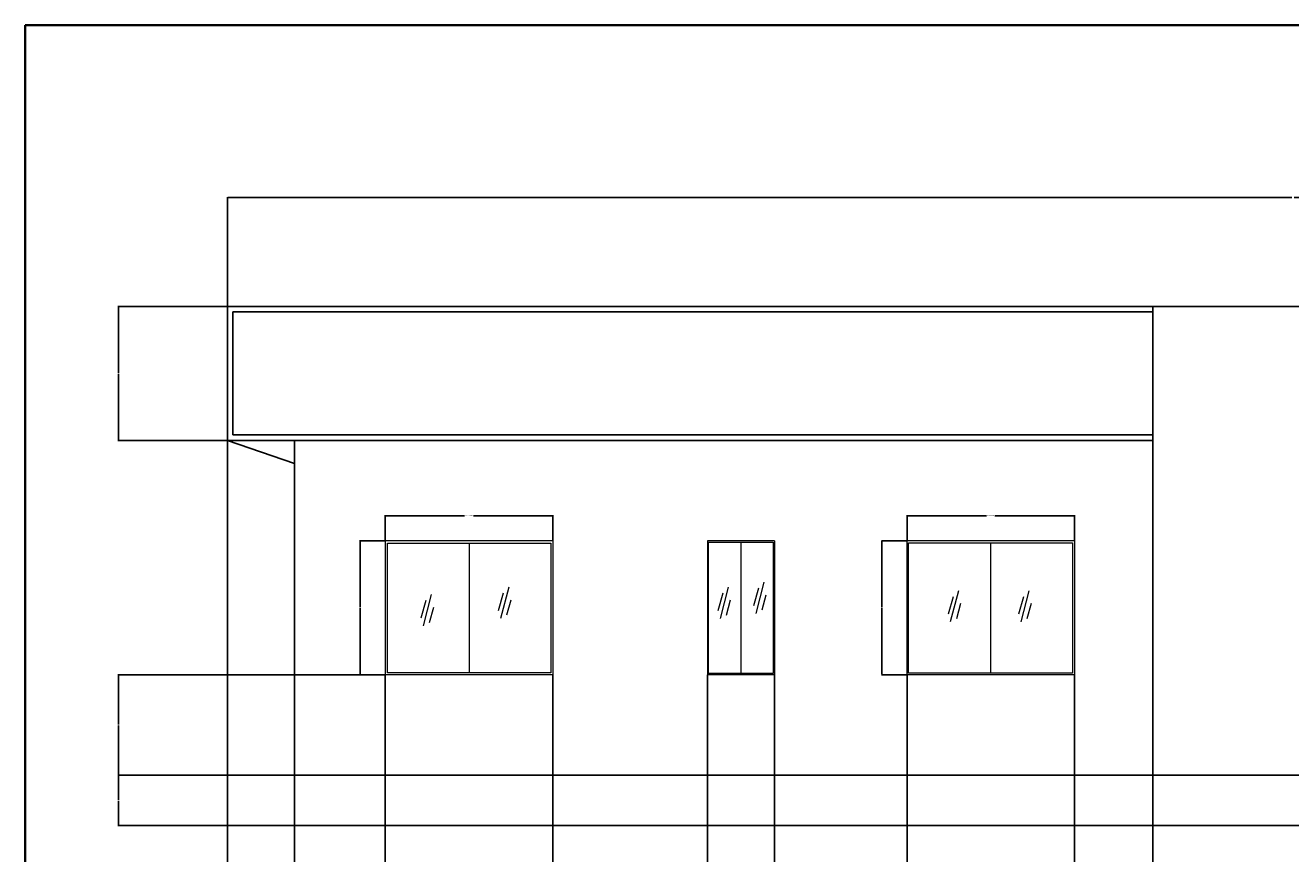
# Model space of a CAD drawing. Units: inches. Extents: x 2314 to 3223, y 1382 to 2735.
# Tile 10 of 14: x 2314 to 2767, y 2439 to 2735. Entities that reach past the tile are written whole.
import ezdxf

# ---------------------------------------------------------------- set-up
doc = ezdxf.new("R2010")
doc.units = ezdxf.units.IN
for name, color, linetype, lineweight in [('A-ANNO-DIMS', 2, 'Continuous', 18), ('A-ANNO-TTLB', 7, 'Continuous', 35), ('A-ELEV', 7, 'Continuous', 25), ('A-GLAZ-ELEV', 4, 'Continuous', 18)]:
    doc.layers.add(name, color=color, linetype=linetype, lineweight=lineweight)
doc.styles.get("Standard").update_dxf_attribs({"font": 'arial.ttf'})
doc.dimstyles.get("Standard").update_dxf_attribs({"dimtxt": 0.18, "dimasz": 0.18, "dimexe": 0.18, "dimexo": 0.0625, "dimgap": 0.09, "dimtad": 0, "dimtih": 1, "dimtoh": 1, "dimdec": 4, "dimzin": 0, "dimdsep": 46, "dimtxsty": 'Standard', "dimcen": 0.09, "dimadec": 0, "dimazin": 0, "dimtfac": 1, "dimtdec": 4, "dimtofl": 0, "dimtmove": 0, "dimatfit": 3, "dimfxl": 1, "dimtolj": 1, "dimtzin": 0, "dimarcsym": 0})

# ---------------------------------------------------------------- blocks, each defined once
blk = doc.blocks.new('WIN-ELEV-60X48-DIVIDED')
for p, q in [((0, 48), (0, 0)), ((60, 48), (0, 48)), ((30.07, 47.13), (30.07, 0.71)), ((60, 48), (60, 0)), ((60, 0), (0, 0))]:
    blk.add_line(p, q)
blk.add_lwpolyline([(0.83, 47.13), (59.31, 47.13), (59.31, 0.71), (0.83, 0.71)], close=True)
blk = doc.blocks.new('WIN-ELEV-60X48-FRAME-SASH')
for p, q in [((0, 48), (0, 0)), ((60, 48), (0, 48)), ((60, 48), (60, 0)), ((60, 0), (0, 0))]:
    blk.add_line(p, q)
blk.add_lwpolyline([(0.54, 47.23), (59.34, 47.23), (59.34, 0.63), (0.54, 0.63)], close=True)
blk = doc.blocks.new('WIN-ELEV-24X48-FRAME')
for p, q in [((0, 48), (0, 0)), ((24, 48), (0, 48)), ((24, 48), (24, 0)), ((24, 0), (0, 0))]:
    blk.add_line(p, q)
blk = doc.blocks.new('GLASS-REFLECTION-MARK')
for p, q in [((3.77, 11.17), (0.81, 0)), ((1.83, 9.04), (0, 2.74)), ((4.5, 6.57), (2.99, 1.12))]:
    blk.add_line(p, q)
blk = doc.blocks.new('*D21')
at = {"layer": 'A-ANNO-DIMS', "color": 0, "lineweight": -2, "transparency": 16777216}
for p, q in [((2442.93, 2550.74), (2442.93, 2559.86)), ((2443.11, 2559.68), (2471.28, 2559.68)), ((2502.75, 2559.68), (2474.59, 2559.68)), ((2502.93, 2550.74), (2502.93, 2559.86))]:
    blk.add_line(p, q, dxfattribs=at)
at = {"layer": 'A-ANNO-DIMS', "color": 0, "transparency": 16777216}
for points in [[(2443.11, 2559.71), (2443.11, 2559.65), (2442.93, 2559.68)], [(2502.75, 2559.71), (2502.75, 2559.65), (2502.93, 2559.68)]]:
    blk.add_solid(points, dxfattribs=at)
at = {"layer": 'Defpoints', "color": 0, "transparency": 16777216}
for p in [(2502.93, 2559.68), (2442.93, 2550.68), (2502.93, 2550.68)]:
    blk.add_point(p, dxfattribs=at)
at = {"layer": 'A-ANNO-DIMS', "color": 0, "transparency": 16777216, "insert": (2472.93, 2559.68), "char_height": 0.18, "attachment_point": 5}
blk.add_mtext('\\A1;DIVIDED WINDOW 60 TYP.', dxfattribs=at)
blk = doc.blocks.new('*D22')
at = {"layer": 'A-ANNO-DIMS', "color": 0, "lineweight": -2, "transparency": 16777216}
for p, q in [((2442.87, 2550.68), (2433.75, 2550.68)), ((2433.93, 2550.5), (2433.93, 2526.86)), ((2433.93, 2502.86), (2433.93, 2526.5)), ((2442.87, 2502.68), (2433.75, 2502.68))]:
    blk.add_line(p, q, dxfattribs=at)
at = {"layer": 'A-ANNO-DIMS', "color": 0, "transparency": 16777216}
for points in [[(2433.9, 2550.5), (2433.96, 2550.5), (2433.93, 2550.68)], [(2433.9, 2502.86), (2433.96, 2502.86), (2433.93, 2502.68)]]:
    blk.add_solid(points, dxfattribs=at)
at = {"layer": 'Defpoints', "color": 0, "transparency": 16777216}
for p in [(2433.93, 2550.68), (2442.93, 2550.68), (2442.93, 2502.68)]:
    blk.add_point(p, dxfattribs=at)
at = {"layer": 'A-ANNO-DIMS', "color": 0, "transparency": 16777216, "insert": (2433.93, 2526.68), "char_height": 0.18, "attachment_point": 5}
blk.add_mtext('\\A1;48 TYP.', dxfattribs=at)
blk = doc.blocks.new('*D23')
at = {"layer": 'A-ANNO-DIMS', "color": 0, "lineweight": -2, "transparency": 16777216}
for p, q in [((2629.85, 2550.74), (2629.85, 2559.86)), ((2630.03, 2559.68), (2658.35, 2559.68)), ((2689.67, 2559.68), (2661.34, 2559.68)), ((2689.85, 2550.74), (2689.85, 2559.86))]:
    blk.add_line(p, q, dxfattribs=at)
at = {"layer": 'A-ANNO-DIMS', "color": 0, "transparency": 16777216}
for points in [[(2630.03, 2559.71), (2630.03, 2559.65), (2629.85, 2559.68)], [(2689.67, 2559.71), (2689.67, 2559.65), (2689.85, 2559.68)]]:
    blk.add_solid(points, dxfattribs=at)
at = {"layer": 'Defpoints', "color": 0, "transparency": 16777216}
for p in [(2689.85, 2559.68), (2629.85, 2550.68), (2689.85, 2550.68)]:
    blk.add_point(p, dxfattribs=at)
at = {"layer": 'A-ANNO-DIMS', "color": 0, "transparency": 16777216, "insert": (2659.85, 2559.68), "char_height": 0.18, "attachment_point": 5}
blk.add_mtext('\\A1;WINDOW SASH 60 TYP.', dxfattribs=at)
blk = doc.blocks.new('*D24')
at = {"layer": 'A-ANNO-DIMS', "color": 0, "lineweight": -2, "transparency": 16777216}
for p, q in [((2629.78, 2550.68), (2620.67, 2550.68)), ((2620.85, 2550.5), (2620.85, 2526.86)), ((2620.85, 2502.86), (2620.85, 2526.5)), ((2629.78, 2502.68), (2620.67, 2502.68))]:
    blk.add_line(p, q, dxfattribs=at)
at = {"layer": 'A-ANNO-DIMS', "color": 0, "transparency": 16777216}
for points in [[(2620.82, 2550.5), (2620.88, 2550.5), (2620.85, 2550.68)], [(2620.82, 2502.86), (2620.88, 2502.86), (2620.85, 2502.68)]]:
    blk.add_solid(points, dxfattribs=at)
at = {"layer": 'Defpoints', "color": 0, "transparency": 16777216}
for p in [(2620.85, 2550.68), (2629.85, 2550.68), (2629.85, 2502.68)]:
    blk.add_point(p, dxfattribs=at)
at = {"layer": 'A-ANNO-DIMS', "color": 0, "transparency": 16777216, "insert": (2620.85, 2526.68), "char_height": 0.18, "attachment_point": 5}
blk.add_mtext('\\A1;48 TYP.', dxfattribs=at)
blk = doc.blocks.new('*D46')
at = {"layer": 'A-ANNO-DIMS', "color": 0, "lineweight": -2, "transparency": 16777216}
for p, q in [((2386.39, 2634.74), (2386.39, 2673.86)), ((2386.57, 2673.68), (2767.75, 2673.68)), ((3149.71, 2673.68), (2768.54, 2673.68)), ((3149.89, 2634.74), (3149.89, 2673.86))]:
    blk.add_line(p, q, dxfattribs=at)
at = {"layer": 'A-ANNO-DIMS', "color": 0, "transparency": 16777216}
for points in [[(2386.57, 2673.71), (2386.57, 2673.65), (2386.39, 2673.68)], [(3149.71, 2673.71), (3149.71, 2673.65), (3149.89, 2673.68)]]:
    blk.add_solid(points, dxfattribs=at)
at = {"layer": 'Defpoints', "color": 0, "transparency": 16777216}
for p in [(3149.89, 2673.68), (2386.39, 2634.68), (3149.89, 2634.68)]:
    blk.add_point(p, dxfattribs=at)
at = {"layer": 'A-ANNO-DIMS', "color": 0, "transparency": 16777216, "insert": (2768.14, 2673.68), "char_height": 0.18, "attachment_point": 5}
blk.add_mtext('\\A1;763.5', dxfattribs=at)
blk = doc.blocks.new('*D48')
at = {"layer": 'A-ANNO-DIMS', "color": 0, "lineweight": -2, "transparency": 16777216}
for p, q in [((2442.87, 2502.68), (2347.21, 2502.68)), ((2347.39, 2502.5), (2347.39, 2484.86)), ((2347.39, 2466.86), (2347.39, 2484.5)), ((2410.33, 2466.68), (2347.21, 2466.68))]:
    blk.add_line(p, q, dxfattribs=at)
at = {"layer": 'A-ANNO-DIMS', "color": 0, "transparency": 16777216}
for points in [[(2347.36, 2502.5), (2347.42, 2502.5), (2347.39, 2502.68)], [(2347.36, 2466.86), (2347.42, 2466.86), (2347.39, 2466.68)]]:
    blk.add_solid(points, dxfattribs=at)
at = {"layer": 'Defpoints', "color": 0, "transparency": 16777216}
for p in [(2347.39, 2502.68), (2442.93, 2502.68), (2410.39, 2466.68)]:
    blk.add_point(p, dxfattribs=at)
at = {"layer": 'A-ANNO-DIMS', "color": 0, "transparency": 16777216, "insert": (2347.39, 2484.68), "char_height": 0.18, "attachment_point": 5}
blk.add_mtext('\\A1;36', dxfattribs=at)
blk = doc.blocks.new('*D49')
at = {"layer": 'A-ANNO-DIMS', "color": 0, "lineweight": -2, "transparency": 16777216}
for p, q in [((2410.33, 2466.68), (2347.21, 2466.68)), ((2347.39, 2466.5), (2347.39, 2457.86)), ((2347.39, 2448.86), (2347.39, 2457.5)), ((2410.33, 2448.68), (2347.21, 2448.68))]:
    blk.add_line(p, q, dxfattribs=at)
at = {"layer": 'A-ANNO-DIMS', "color": 0, "transparency": 16777216}
for points in [[(2347.36, 2466.5), (2347.42, 2466.5), (2347.39, 2466.68)], [(2347.36, 2448.86), (2347.42, 2448.86), (2347.39, 2448.68)]]:
    blk.add_solid(points, dxfattribs=at)
at = {"layer": 'Defpoints', "color": 0, "transparency": 16777216}
for p in [(2410.39, 2466.68), (2347.39, 2448.68), (2410.39, 2448.68)]:
    blk.add_point(p, dxfattribs=at)
at = {"layer": 'A-ANNO-DIMS', "color": 0, "transparency": 16777216, "insert": (2347.39, 2457.68), "char_height": 0.18, "attachment_point": 5}
blk.add_mtext('\\A1;18', dxfattribs=at)
blk = doc.blocks.new('*D50')
at = {"layer": 'A-ANNO-DIMS', "color": 0, "lineweight": -2, "transparency": 16777216}
for p, q in [((2386.33, 2634.68), (2347.21, 2634.68)), ((2347.39, 2634.5), (2347.39, 2610.86)), ((2347.39, 2586.86), (2347.39, 2610.5)), ((2386.33, 2586.68), (2347.21, 2586.68))]:
    blk.add_line(p, q, dxfattribs=at)
at = {"layer": 'A-ANNO-DIMS', "color": 0, "transparency": 16777216}
for points in [[(2347.36, 2634.5), (2347.42, 2634.5), (2347.39, 2634.68)], [(2347.36, 2586.86), (2347.42, 2586.86), (2347.39, 2586.68)]]:
    blk.add_solid(points, dxfattribs=at)
at = {"layer": 'Defpoints', "color": 0, "transparency": 16777216}
for p in [(2386.39, 2634.68), (2347.39, 2586.68), (2386.39, 2586.68)]:
    blk.add_point(p, dxfattribs=at)
at = {"layer": 'A-ANNO-DIMS', "color": 0, "transparency": 16777216, "insert": (2347.39, 2610.68), "char_height": 0.18, "attachment_point": 5}
blk.add_mtext('\\A1;48', dxfattribs=at)
blk = doc.blocks.new('*D51')
at = {"layer": 'A-ANNO-DIMS', "color": 0, "lineweight": -2, "transparency": 16777216}
for p, q in [((2386.39, 2586.62), (2386.39, 2371.63)), ((2410.39, 2578.28), (2410.39, 2371.63)), ((2386.57, 2371.81), (2398.17, 2371.81)), ((2410.21, 2371.81), (2398.61, 2371.81))]:
    blk.add_line(p, q, dxfattribs=at)
at = {"layer": 'A-ANNO-DIMS', "color": 0, "transparency": 16777216}
for points in [[(2386.57, 2371.84), (2386.57, 2371.78), (2386.39, 2371.81)], [(2410.21, 2371.84), (2410.21, 2371.78), (2410.39, 2371.81)]]:
    blk.add_solid(points, dxfattribs=at)
at = {"layer": 'Defpoints', "color": 0, "transparency": 16777216}
for p in [(2386.39, 2586.68), (2410.39, 2578.34), (2410.39, 2371.81)]:
    blk.add_point(p, dxfattribs=at)
at = {"layer": 'A-ANNO-DIMS', "color": 0, "transparency": 16777216, "insert": (2398.39, 2371.81), "char_height": 0.18, "attachment_point": 5}
blk.add_mtext('\\A1;24', dxfattribs=at)
blk = doc.blocks.new('*D52')
at = {"layer": 'A-ANNO-DIMS', "color": 0, "lineweight": -2, "transparency": 16777216}
for p, q in [((2442.93, 2502.62), (2442.93, 2371.63)), ((2410.39, 2466.62), (2410.39, 2371.63)), ((2410.57, 2371.81), (2426.27, 2371.81)), ((2442.75, 2371.81), (2427.06, 2371.81))]:
    blk.add_line(p, q, dxfattribs=at)
at = {"layer": 'A-ANNO-DIMS', "color": 0, "transparency": 16777216}
for points in [[(2410.57, 2371.84), (2410.57, 2371.78), (2410.39, 2371.81)], [(2442.75, 2371.84), (2442.75, 2371.78), (2442.93, 2371.81)]]:
    blk.add_solid(points, dxfattribs=at)
at = {"layer": 'Defpoints', "color": 0, "transparency": 16777216}
for p in [(2442.93, 2502.68), (2410.39, 2466.68), (2442.93, 2371.81)]:
    blk.add_point(p, dxfattribs=at)
at = {"layer": 'A-ANNO-DIMS', "color": 0, "transparency": 16777216, "insert": (2426.66, 2371.81), "char_height": 0.18, "attachment_point": 5}
blk.add_mtext('\\A1;32.54', dxfattribs=at)
blk = doc.blocks.new('*D53')
at = {"layer": 'A-ANNO-DIMS', "color": 0, "lineweight": -2, "transparency": 16777216}
for p, q in [((2502.93, 2502.62), (2502.93, 2371.63)), ((2558.38, 2502.62), (2558.38, 2371.63)), ((2503.11, 2371.81), (2530.26, 2371.81)), ((2558.2, 2371.81), (2531.05, 2371.81))]:
    blk.add_line(p, q, dxfattribs=at)
at = {"layer": 'A-ANNO-DIMS', "color": 0, "transparency": 16777216}
for points in [[(2503.11, 2371.84), (2503.11, 2371.78), (2502.93, 2371.81)], [(2558.2, 2371.84), (2558.2, 2371.78), (2558.38, 2371.81)]]:
    blk.add_solid(points, dxfattribs=at)
at = {"layer": 'Defpoints', "color": 0, "transparency": 16777216}
for p in [(2502.93, 2502.68), (2558.38, 2502.68), (2558.38, 2371.81)]:
    blk.add_point(p, dxfattribs=at)
at = {"layer": 'A-ANNO-DIMS', "color": 0, "transparency": 16777216, "insert": (2530.66, 2371.81), "char_height": 0.18, "attachment_point": 5}
blk.add_mtext('\\A1;55.45', dxfattribs=at)
blk = doc.blocks.new('*D54')
at = {"layer": 'A-ANNO-DIMS', "color": 0, "lineweight": -2, "transparency": 16777216}
for p, q in [((2582.38, 2502.62), (2582.38, 2371.63)), ((2629.85, 2502.62), (2629.85, 2371.63)), ((2582.56, 2371.81), (2605.72, 2371.81)), ((2629.67, 2371.81), (2606.51, 2371.81))]:
    blk.add_line(p, q, dxfattribs=at)
at = {"layer": 'A-ANNO-DIMS', "color": 0, "transparency": 16777216}
for points in [[(2582.56, 2371.84), (2582.56, 2371.78), (2582.38, 2371.81)], [(2629.67, 2371.84), (2629.67, 2371.78), (2629.85, 2371.81)]]:
    blk.add_solid(points, dxfattribs=at)
at = {"layer": 'Defpoints', "color": 0, "transparency": 16777216}
for p in [(2582.38, 2502.68), (2629.85, 2502.68), (2629.85, 2371.81)]:
    blk.add_point(p, dxfattribs=at)
at = {"layer": 'A-ANNO-DIMS', "color": 0, "transparency": 16777216, "insert": (2606.11, 2371.81), "char_height": 0.18, "attachment_point": 5}
blk.add_mtext('\\A1;47.47', dxfattribs=at)
blk = doc.blocks.new('*D55')
at = {"layer": 'A-ANNO-DIMS', "color": 0, "lineweight": -2, "transparency": 16777216}
for p, q in [((2689.85, 2502.62), (2689.85, 2371.63)), ((2717.89, 2466.62), (2717.89, 2371.63)), ((2690.03, 2371.81), (2703.4, 2371.81)), ((2717.71, 2371.81), (2704.33, 2371.81))]:
    blk.add_line(p, q, dxfattribs=at)
at = {"layer": 'A-ANNO-DIMS', "color": 0, "transparency": 16777216}
for points in [[(2690.03, 2371.84), (2690.03, 2371.78), (2689.85, 2371.81)], [(2717.71, 2371.84), (2717.71, 2371.78), (2717.89, 2371.81)]]:
    blk.add_solid(points, dxfattribs=at)
at = {"layer": 'Defpoints', "color": 0, "transparency": 16777216}
for p in [(2689.85, 2502.68), (2717.89, 2466.68), (2717.89, 2371.81)]:
    blk.add_point(p, dxfattribs=at)
at = {"layer": 'A-ANNO-DIMS', "color": 0, "transparency": 16777216, "insert": (2703.87, 2371.81), "char_height": 0.18, "attachment_point": 5}
blk.add_mtext('\\A1;28.046', dxfattribs=at)
blk = doc.blocks.new('*D56')
at = {"layer": 'A-ANNO-DIMS', "color": 0, "lineweight": -2, "transparency": 16777216}
for p, q in [((2717.89, 2466.62), (2717.89, 2371.63)), ((2822.89, 2466.62), (2822.89, 2371.63)), ((2718.07, 2371.81), (2770.11, 2371.81)), ((2822.71, 2371.81), (2770.67, 2371.81))]:
    blk.add_line(p, q, dxfattribs=at)
at = {"layer": 'A-ANNO-DIMS', "color": 0, "transparency": 16777216}
for points in [[(2718.07, 2371.84), (2718.07, 2371.78), (2717.89, 2371.81)], [(2822.71, 2371.84), (2822.71, 2371.78), (2822.89, 2371.81)]]:
    blk.add_solid(points, dxfattribs=at)
at = {"layer": 'Defpoints', "color": 0, "transparency": 16777216}
for p in [(2717.89, 2466.68), (2822.89, 2466.68), (2822.89, 2371.81)]:
    blk.add_point(p, dxfattribs=at)
at = {"layer": 'A-ANNO-DIMS', "color": 0, "transparency": 16777216, "insert": (2770.39, 2371.81), "char_height": 0.18, "attachment_point": 5}
blk.add_mtext('\\A1;105', dxfattribs=at)

msp = doc.modelspace()

# ---------------------------------------------------------------- linework, layer by layer
at = {"layer": 'A-ANNO-TTLB'}
msp.add_lwpolyline([(2314.008, 2735.417), (3222.6676, 2735.417), (3222.6676, 1382.0876), (2314.008, 1382.0876)], close=True, dxfattribs=at)
at = {"layer": 'A-ELEV'}
for p, q in [((3149.8927, 2634.6793), (2386.3927, 2634.6793)), ((2386.3927, 2586.6793), (2386.3927, 2634.6793)), ((2386.3927, 2634.6793), (2386.3927, 2632.6793)), ((2717.8927, 2586.6793), (2717.8927, 2634.6793)), ((2388.3927, 2632.6793), (2717.8927, 2632.6793)), ((2388.3927, 2588.6793), (2388.3927, 2632.6793)), ((2717.8927, 2588.6793), (2388.3927, 2588.6793)), ((2717.8927, 2586.6793), (2386.3927, 2586.6793)), ((2386.3927, 2586.6793), (2410.3927, 2578.3383)), ((2410.3927, 2586.6793), (2410.3927, 2448.6793)), ((2717.8927, 2586.6793), (2717.8927, 2466.6793)), ((3125.8927, 2466.6793), (2410.3927, 2466.6793)), ((3125.8927, 2448.6793), (2410.3927, 2448.6793))]:
    msp.add_line(p, q, dxfattribs=at)
at = {"layer": 'A-GLAZ-ELEV'}
for p, q in [((2570.3329, 2550.2273), (2570.3329, 2503.1249)), ((2659.7868, 2549.9127), (2659.7868, 2503.3075))]:
    msp.add_line(p, q, dxfattribs=at)
msp.add_lwpolyline([(2558.7563, 2550.2273), (2581.9095, 2550.2273), (2581.9095, 2503.1249), (2558.7563, 2503.1249)], close=True, dxfattribs=at)

# ---------------------------------------------------------------- block references
for name, p in [('WIN-ELEV-60X48-DIVIDED', (2442.9339, 2502.6793)), ('WIN-ELEV-24X48-FRAME', (2558.3793, 2502.6793)), ('WIN-ELEV-60X48-FRAME-SASH', (2629.8467, 2502.6793)), ('GLASS-REFLECTION-MARK', (2483.412, 2522.8895)), ('GLASS-REFLECTION-MARK', (2562.0549, 2522.8424)), ('GLASS-REFLECTION-MARK', (2574.8382, 2524.6934)), ('GLASS-REFLECTION-MARK', (2455.6851, 2520.2246)), ('GLASS-REFLECTION-MARK', (2644.5429, 2521.6088)), ('GLASS-REFLECTION-MARK', (2669.7739, 2521.6088))]:
    msp.add_blockref(name, p, dxfattribs=at)

# ---------------------------------------------------------------- dimensions: what is measured, and where the dimension line sits
at = {"layer": 'A-ANNO-DIMS'}
for base, p1, p2, override, picture, middle in [((3149.8927, 2673.6793), (2386.3927, 2634.6793), (3149.8927, 2634.6793), {"dimdec": 1, "dimlfac": 1, "dimrnd": 0, "dimzin": 0, "dimdsep": 46, "dimlunit": 2}, '*D46', (2768.1427, 2673.6793)), ((2410.3927, 2371.8121), (2386.3927, 2586.6793), (2410.3927, 2578.3383), {"dimdec": 0, "dimlfac": 1, "dimrnd": 0, "dimzin": 0, "dimdsep": 46, "dimlunit": 2}, '*D51', (2398.3927, 2371.8121)), ((2442.9339, 2371.8121), (2410.3927, 2466.6793), (2442.9339, 2502.6793), {"dimdec": 2, "dimlfac": 1, "dimrnd": 0, "dimzin": 0, "dimdsep": 46, "dimlunit": 2}, '*D52', (2426.6633, 2371.8121)), ((2558.3793, 2371.8121), (2502.9339, 2502.6793), (2558.3793, 2502.6793), {"dimdec": 2, "dimlfac": 1, "dimrnd": 0, "dimzin": 0, "dimdsep": 46, "dimlunit": 2}, '*D53', (2530.6566, 2371.8121)), ((2629.8467, 2371.8121), (2582.3793, 2502.6793), (2629.8467, 2502.6793), {"dimdec": 2, "dimlfac": 1, "dimrnd": 0, "dimzin": 0, "dimdsep": 46, "dimlunit": 2}, '*D54', (2606.113, 2371.8121)), ((2717.8927, 2371.8121), (2689.8467, 2502.6793), (2717.8927, 2466.6793), {"dimdec": 3, "dimlfac": 1, "dimrnd": 0, "dimzin": 0, "dimdsep": 46, "dimlunit": 2}, '*D55', (2703.8697, 2371.8121)), ((2822.8927, 2371.8121), (2717.8927, 2466.6793), (2822.8927, 2466.6793), {"dimdec": 0, "dimlfac": 1, "dimrnd": 0, "dimzin": 0, "dimdsep": 46, "dimlunit": 2}, '*D56', (2770.3927, 2371.8121))]:
    dim = msp.add_linear_dim(base=base, p1=p1, p2=p2, dimstyle='Standard', override=override, dxfattribs=at)
    dim.commit()
    dim.dimension.update_dxf_attribs({"geometry": picture, "text_midpoint": middle})
for base, p1, p2, picture, middle in [((2347.3927, 2586.6793), (2386.3927, 2634.6793), (2386.3927, 2586.6793), '*D50', (2347.3927, 2610.6793)), ((2347.3927, 2502.6793), (2410.3927, 2466.6793), (2442.9339, 2502.6793), '*D48', (2347.3927, 2484.6793)), ((2347.3927, 2448.6793), (2410.3927, 2466.6793), (2410.3927, 2448.6793), '*D49', (2347.3927, 2457.6793))]:
    dim = msp.add_linear_dim(base=base, p1=p1, p2=p2, angle=90, dimstyle='Standard', override={"dimdec": 0, "dimlfac": 1, "dimrnd": 0, "dimzin": 0, "dimdsep": 46, "dimlunit": 2}, dxfattribs=at)
    dim.commit()
    dim.dimension.update_dxf_attribs({"geometry": picture, "text_midpoint": middle})
for base, p1, p2, text, picture, middle in [((2502.9339, 2559.6793), (2442.9339, 2550.6793), (2502.9339, 2550.6793), 'DIVIDED WINDOW <> TYP.', '*D21', (2472.9339, 2559.6793)), ((2689.8467, 2559.6793), (2629.8467, 2550.6793), (2689.8467, 2550.6793), 'WINDOW SASH <> TYP.', '*D23', (2659.8467, 2559.6793))]:
    dim = msp.add_linear_dim(base=base, p1=p1, p2=p2, text=text, dimstyle='Standard', override={"dimdec": 0, "dimlfac": 1, "dimrnd": 0, "dimzin": 0, "dimdsep": 46, "dimlunit": 2}, dxfattribs=at)
    dim.commit()
    dim.dimension.update_dxf_attribs({"geometry": picture, "text_midpoint": middle})
for base, p1, p2, picture, middle in [((2433.9339, 2550.6793), (2442.9339, 2502.6793), (2442.9339, 2550.6793), '*D22', (2433.9339, 2526.6793)), ((2620.8467, 2550.6793), (2629.8467, 2502.6793), (2629.8467, 2550.6793), '*D24', (2620.8467, 2526.6793))]:
    dim = msp.add_linear_dim(base=base, p1=p1, p2=p2, angle=90, text='<> TYP.', dimstyle='Standard', override={"dimdec": 0, "dimlfac": 1, "dimrnd": 0, "dimzin": 0, "dimdsep": 46, "dimlunit": 2}, dxfattribs=at)
    dim.commit()
    dim.dimension.update_dxf_attribs({"geometry": picture, "text_midpoint": middle})

doc.saveas('drawing.dxf')
